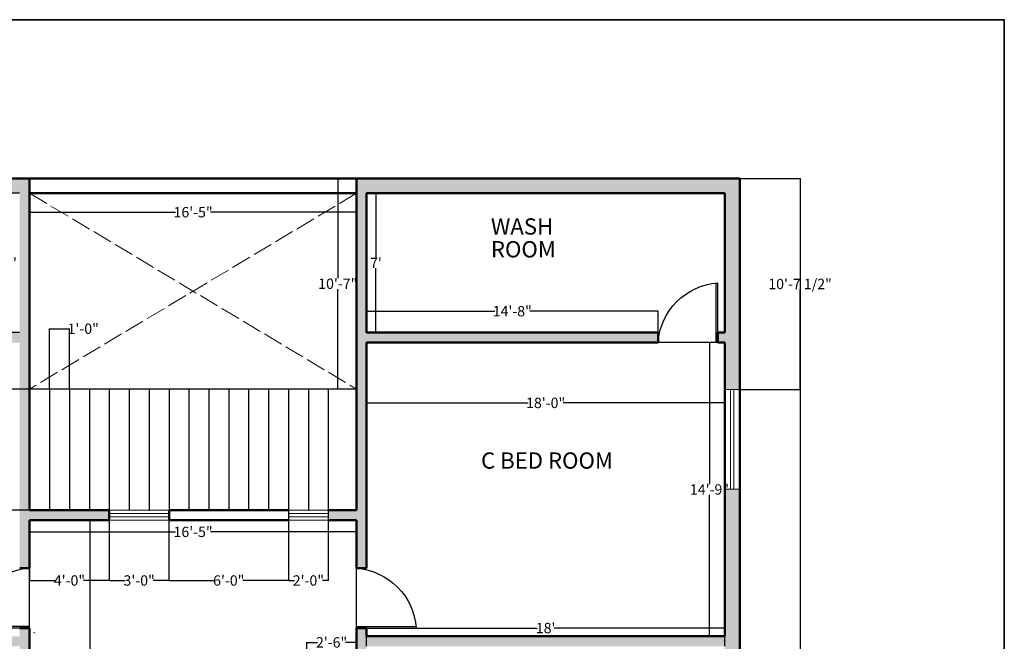
# Model space of a CAD drawing. Units: inches. Extents: x -335 to 1312, y -66 to 821.
# Tile 4 of 4: x 719 to 1312, y 446 to 821. Entities that reach past the tile are written whole.
import ezdxf

# ---------------------------------------------------------------- set-up
doc = ezdxf.new("R2010")
doc.units = ezdxf.units.IN
doc.header["$MEASUREMENT"] = 0
doc.linetypes.add('ACAD_ISO02W100', pattern=[15, 12, -3])
for name, color, linetype, lineweight in [('A-ANNO-DIMS', 2, 'Continuous', 18), ('A-ANNO-TTLB', 7, 'Continuous', 35), ('A-AREA-IDEN', 7, 'Continuous', 25), ('A-DOOR', 34, 'Continuous', 25), ('A-FLOR-OVHD', 8, 'ACAD_ISO02W100', 13), ('A-FLOR-STRS', 7, 'Continuous', 25), ('A-GLAZ', 34, 'Continuous', 18), ('A-WALL', 7, 'Continuous', 50), ('A-WALL-PATT', 252, 'Continuous', 13)]:
    doc.layers.add(name, color=color, linetype=linetype, lineweight=lineweight)
doc.styles.get("Standard").update_dxf_attribs({"font": 'arial.ttf'})
doc.dimstyles.get("Standard").update_dxf_attribs({"dimtxt": 6.25, "dimasz": 0.18, "dimexe": 0.18, "dimexo": 0.0625, "dimgap": 0.09, "dimtad": 0, "dimtih": 1, "dimtoh": 1, "dimdec": 0, "dimzin": 0, "dimdsep": 46, "dimlunit": 3, "dimtxsty": 'Standard', "dimcen": 0.09, "dimadec": 0, "dimazin": 0, "dimtfac": 1, "dimtdec": 0, "dimtofl": 0, "dimtmove": 0, "dimatfit": 3, "dimfxl": 1, "dimtolj": 1, "dimtzin": 0, "dimarcsym": 0})

# ---------------------------------------------------------------- blocks, each defined once
blk = doc.blocks.new('*D2')
at = {"layer": 'A-ANNO-DIMS', "color": 0, "lineweight": -2, "transparency": 16777216}
for p, q in [((718.49, 716.41), (713.15, 716.41)), ((713.33, 716.23), (713.33, 677.62)), ((713.33, 632.59), (713.33, 671.19)), ((718.49, 632.41), (713.15, 632.41))]:
    blk.add_line(p, q, dxfattribs=at)
at = {"layer": 'A-ANNO-DIMS', "color": 0, "transparency": 16777216}
for points in [[(713.3, 716.23), (713.36, 716.23), (713.33, 716.41)], [(713.3, 632.59), (713.36, 632.59), (713.33, 632.41)]]:
    blk.add_solid(points, dxfattribs=at)
at = {"layer": 'Defpoints', "color": 0, "transparency": 16777216}
for p in [(718.55, 716.41), (713.33, 632.41), (718.55, 632.41)]:
    blk.add_point(p, dxfattribs=at)
at = {"layer": 'A-ANNO-DIMS', "color": 0, "transparency": 16777216, "insert": (713.33, 674.41), "char_height": 6.25, "attachment_point": 5}
blk.add_mtext("\\A1;7'", dxfattribs=at)
blk = doc.blocks.new('*D18')
at = {"layer": 'A-ANNO-DIMS', "color": 0, "lineweight": -2, "transparency": 16777216}
for p, q in [((927.55, 443.47), (927.55, 454.59)), ((927.73, 454.41), (1030.45, 454.41)), ((1143.37, 454.41), (1040.65, 454.41)), ((1143.55, 443.47), (1143.55, 454.59))]:
    blk.add_line(p, q, dxfattribs=at)
at = {"layer": 'A-ANNO-DIMS', "color": 0, "transparency": 16777216}
for points in [[(927.73, 454.44), (927.73, 454.38), (927.55, 454.41)], [(1143.37, 454.44), (1143.37, 454.38), (1143.55, 454.41)]]:
    blk.add_solid(points, dxfattribs=at)
at = {"layer": 'Defpoints', "color": 0, "transparency": 16777216}
for p in [(927.55, 454.41), (927.55, 443.41), (1143.55, 443.41)]:
    blk.add_point(p, dxfattribs=at)
at = {"layer": 'A-ANNO-DIMS', "color": 0, "transparency": 16777216, "insert": (1035.55, 454.41), "char_height": 6.25, "attachment_point": 5}
blk.add_mtext("\\A1;18'", dxfattribs=at)
blk = doc.blocks.new('*D19')
at = {"layer": 'A-ANNO-DIMS', "color": 0, "lineweight": -2, "transparency": 16777216}
for p, q in [((1143.49, 626.41), (1134.12, 626.41)), ((1134.3, 626.23), (1134.3, 541.19)), ((1134.3, 449.59), (1134.3, 534.63)), ((1143.49, 449.41), (1134.12, 449.41))]:
    blk.add_line(p, q, dxfattribs=at)
at = {"layer": 'A-ANNO-DIMS', "color": 0, "transparency": 16777216}
for points in [[(1134.27, 626.23), (1134.33, 626.23), (1134.3, 626.41)], [(1134.27, 449.59), (1134.33, 449.59), (1134.3, 449.41)]]:
    blk.add_solid(points, dxfattribs=at)
at = {"layer": 'Defpoints', "color": 0, "transparency": 16777216}
for p in [(1134.3, 626.41), (1143.55, 626.41), (1143.55, 449.41)]:
    blk.add_point(p, dxfattribs=at)
at = {"layer": 'A-ANNO-DIMS', "color": 0, "transparency": 16777216, "insert": (1134.3, 537.91), "char_height": 6.25, "attachment_point": 5}
blk.add_mtext('\\A1;14\'-9"', dxfattribs=at)
blk = doc.blocks.new('*D20')
at = {"layer": 'A-ANNO-DIMS', "color": 0, "lineweight": -2, "transparency": 16777216}
for p, q in [((927.55, 632.47), (927.55, 645.55)), ((927.73, 645.37), (1004.9, 645.37)), ((1103.13, 645.37), (1025.96, 645.37)), ((1103.31, 632.47), (1103.31, 645.55))]:
    blk.add_line(p, q, dxfattribs=at)
at = {"layer": 'A-ANNO-DIMS', "color": 0, "transparency": 16777216}
for points in [[(927.73, 645.4), (927.73, 645.34), (927.55, 645.37)], [(1103.13, 645.4), (1103.13, 645.34), (1103.31, 645.37)]]:
    blk.add_solid(points, dxfattribs=at)
at = {"layer": 'Defpoints', "color": 0, "transparency": 16777216}
for p in [(927.55, 645.37), (927.55, 632.41), (1103.31, 632.41)]:
    blk.add_point(p, dxfattribs=at)
at = {"layer": 'A-ANNO-DIMS', "color": 0, "transparency": 16777216, "insert": (1015.43, 645.37), "char_height": 6.25, "attachment_point": 5}
blk.add_mtext('\\A1;14\'-8"', dxfattribs=at)
blk = doc.blocks.new('*D21')
at = {"layer": 'A-ANNO-DIMS', "color": 0, "lineweight": -2, "transparency": 16777216}
for p, q in [((927.61, 716.41), (933.44, 716.41)), ((933.26, 716.23), (933.26, 677.62)), ((933.26, 632.59), (933.26, 671.19)), ((927.61, 632.41), (933.44, 632.41))]:
    blk.add_line(p, q, dxfattribs=at)
at = {"layer": 'A-ANNO-DIMS', "color": 0, "transparency": 16777216}
for points in [[(933.23, 716.23), (933.29, 716.23), (933.26, 716.41)], [(933.23, 632.59), (933.29, 632.59), (933.26, 632.41)]]:
    blk.add_solid(points, dxfattribs=at)
at = {"layer": 'Defpoints', "color": 0, "transparency": 16777216}
for p in [(927.55, 716.41), (927.55, 632.41), (933.26, 632.41)]:
    blk.add_point(p, dxfattribs=at)
at = {"layer": 'A-ANNO-DIMS', "color": 0, "transparency": 16777216, "insert": (933.26, 674.41), "char_height": 6.25, "attachment_point": 5}
blk.add_mtext("\\A1;7'", dxfattribs=at)
blk = doc.blocks.new('*D22')
at = {"layer": 'A-ANNO-DIMS', "color": 0, "lineweight": -2, "transparency": 16777216}
for p, q in [((724.55, 519.35), (724.55, 512.18)), ((921.55, 519.35), (921.55, 512.18)), ((724.73, 512.36), (812.52, 512.36)), ((921.37, 512.36), (833.58, 512.36))]:
    blk.add_line(p, q, dxfattribs=at)
at = {"layer": 'A-ANNO-DIMS', "color": 0, "transparency": 16777216}
for points in [[(724.73, 512.39), (724.73, 512.33), (724.55, 512.36)], [(921.37, 512.39), (921.37, 512.33), (921.55, 512.36)]]:
    blk.add_solid(points, dxfattribs=at)
at = {"layer": 'Defpoints', "color": 0, "transparency": 16777216}
for p in [(724.55, 519.41), (921.55, 519.41), (921.55, 512.36)]:
    blk.add_point(p, dxfattribs=at)
at = {"layer": 'A-ANNO-DIMS', "color": 0, "transparency": 16777216, "insert": (823.05, 512.36), "char_height": 6.25, "attachment_point": 5}
blk.add_mtext('\\A1;16\'-5"', dxfattribs=at)
blk = doc.blocks.new('*D23')
at = {"layer": 'A-ANNO-DIMS', "color": 0, "lineweight": -2, "transparency": 16777216}
for p, q in [((724.55, 716.35), (724.55, 704.82)), ((921.55, 716.35), (921.55, 704.82)), ((724.73, 705), (812.52, 705)), ((921.37, 705), (833.58, 705))]:
    blk.add_line(p, q, dxfattribs=at)
at = {"layer": 'A-ANNO-DIMS', "color": 0, "transparency": 16777216}
for points in [[(724.73, 705.03), (724.73, 704.97), (724.55, 705)], [(921.37, 705.03), (921.37, 704.97), (921.55, 705)]]:
    blk.add_solid(points, dxfattribs=at)
at = {"layer": 'Defpoints', "color": 0, "transparency": 16777216}
for p in [(724.55, 716.41), (921.55, 716.41), (724.55, 705)]:
    blk.add_point(p, dxfattribs=at)
at = {"layer": 'A-ANNO-DIMS', "color": 0, "transparency": 16777216, "insert": (823.05, 705), "char_height": 6.25, "attachment_point": 5}
blk.add_mtext('\\A1;16\'-5"', dxfattribs=at)
blk = doc.blocks.new('*D24')
at = {"layer": 'A-ANNO-DIMS', "color": 0, "lineweight": -2, "transparency": 16777216}
for p, q in [((921.49, 725.41), (910.09, 725.41)), ((910.27, 725.23), (910.27, 665.19)), ((910.27, 598.59), (910.27, 658.63)), ((921.49, 598.41), (910.09, 598.41))]:
    blk.add_line(p, q, dxfattribs=at)
at = {"layer": 'A-ANNO-DIMS', "color": 0, "transparency": 16777216}
for points in [[(910.24, 725.23), (910.3, 725.23), (910.27, 725.41)], [(910.24, 598.59), (910.3, 598.59), (910.27, 598.41)]]:
    blk.add_solid(points, dxfattribs=at)
at = {"layer": 'Defpoints', "color": 0, "transparency": 16777216}
for p in [(921.55, 725.41), (910.27, 598.41), (921.55, 598.41)]:
    blk.add_point(p, dxfattribs=at)
at = {"layer": 'A-ANNO-DIMS', "color": 0, "transparency": 16777216, "insert": (910.27, 661.91), "char_height": 6.25, "attachment_point": 5}
blk.add_mtext('\\A1;10\'-7"', dxfattribs=at)
blk = doc.blocks.new('WIN-60IN')
for p, q in [((9, 60), (0, 60)), ((0, 60), (0, 0)), ((3.5, 60), (3.5, 0)), ((5.5, 60), (5.5, 0)), ((9, 0), (9, 60)), ((0, 0), (9, 0))]:
    blk.add_line(p, q)
blk = doc.blocks.new('DOOR-SWING-36IN')
for p, q in [((0, 0), (0, 35.94)), ((1, 0), (1, 35.86)), ((0, 0), (36, 0))]:
    blk.add_line(p, q)
blk.add_arc((-2.68, -2.74), 38.78, 4.05456, 86.03519)
blk = doc.blocks.new('*D32')
at = {"layer": 'A-ANNO-DIMS', "color": 0, "lineweight": -2, "transparency": 16777216}
for p, q in [((927.55, 626.35), (927.55, 589.88)), ((1143.55, 626.35), (1143.55, 589.88)), ((927.73, 590.06), (1025.02, 590.06)), ((1143.37, 590.06), (1046.08, 590.06))]:
    blk.add_line(p, q, dxfattribs=at)
at = {"layer": 'A-ANNO-DIMS', "color": 0, "transparency": 16777216}
for points in [[(927.73, 590.09), (927.73, 590.03), (927.55, 590.06)], [(1143.37, 590.09), (1143.37, 590.03), (1143.55, 590.06)]]:
    blk.add_solid(points, dxfattribs=at)
at = {"layer": 'Defpoints', "color": 0, "transparency": 16777216}
for p in [(927.55, 626.41), (1143.55, 626.41), (927.55, 590.06)]:
    blk.add_point(p, dxfattribs=at)
at = {"layer": 'A-ANNO-DIMS', "color": 0, "transparency": 16777216, "insert": (1035.55, 590.06), "char_height": 6.25, "attachment_point": 5}
blk.add_mtext('\\A1;18\'-0"', dxfattribs=at)
blk = doc.blocks.new('*D34')
at = {"layer": 'A-ANNO-DIMS', "color": 0, "lineweight": -2, "transparency": 16777216}
for p, q in [((736.49, 598.41), (700.02, 598.41)), ((700.2, 598.23), (700.2, 565.19)), ((700.2, 525.59), (700.2, 558.63)), ((736.49, 525.41), (700.02, 525.41))]:
    blk.add_line(p, q, dxfattribs=at)
at = {"layer": 'A-ANNO-DIMS', "color": 0, "transparency": 16777216}
for points in [[(700.17, 598.23), (700.23, 598.23), (700.2, 598.41)], [(700.17, 525.59), (700.23, 525.59), (700.2, 525.41)]]:
    blk.add_solid(points, dxfattribs=at)
at = {"layer": 'Defpoints', "color": 0, "transparency": 16777216}
for p in [(700.2, 598.41), (736.55, 598.41), (736.55, 525.41)]:
    blk.add_point(p, dxfattribs=at)
at = {"layer": 'A-ANNO-DIMS', "color": 0, "transparency": 16777216, "insert": (700.2, 561.91), "char_height": 6.25, "attachment_point": 5}
blk.add_mtext('\\A1;6\'-1"', dxfattribs=at)
blk = doc.blocks.new('*D40')
at = {"layer": 'A-ANNO-DIMS', "color": 0, "lineweight": -2, "transparency": 16777216}
for p, q in [((1152.61, 725.41), (1189.08, 725.41)), ((1188.9, 725.23), (1188.9, 665.06)), ((1188.9, 598.25), (1188.9, 658.42)), ((1152.61, 598.07), (1189.08, 598.07))]:
    blk.add_line(p, q, dxfattribs=at)
at = {"layer": 'A-ANNO-DIMS', "color": 0, "transparency": 16777216}
for points in [[(1188.87, 725.23), (1188.93, 725.23), (1188.9, 725.41)], [(1188.87, 598.25), (1188.93, 598.25), (1188.9, 598.07)]]:
    blk.add_solid(points, dxfattribs=at)
at = {"layer": 'Defpoints', "color": 0, "transparency": 16777216}
for p in [(1152.55, 725.41), (1152.55, 598.07), (1188.9, 598.07)]:
    blk.add_point(p, dxfattribs=at)
at = {"layer": 'A-ANNO-DIMS', "color": 0, "transparency": 16777216, "insert": (1188.9, 661.74), "char_height": 6.25, "attachment_point": 5}
blk.add_mtext('\\A1;10\'-7 1/2"', dxfattribs=at)
blk = doc.blocks.new('*D42')
at = {"layer": 'A-ANNO-DIMS', "color": 0, "lineweight": -2, "transparency": 16777216}
for p, q in [((1152.61, 725.41), (1189.08, 725.41)), ((1188.9, 725.23), (1188.9, 368.69)), ((1188.9, 5.59), (1188.9, 362.13)), ((1152.61, 5.41), (1189.08, 5.41))]:
    blk.add_line(p, q, dxfattribs=at)
at = {"layer": 'A-ANNO-DIMS', "color": 0, "transparency": 16777216}
for points in [[(1188.87, 725.23), (1188.93, 725.23), (1188.9, 725.41)], [(1188.87, 5.59), (1188.93, 5.59), (1188.9, 5.41)]]:
    blk.add_solid(points, dxfattribs=at)
at = {"layer": 'Defpoints', "color": 0, "transparency": 16777216}
for p in [(1152.55, 725.41), (1188.9, 725.41), (1152.55, 5.41)]:
    blk.add_point(p, dxfattribs=at)
at = {"layer": 'A-ANNO-DIMS', "color": 0, "transparency": 16777216, "insert": (1188.9, 365.41), "char_height": 6.25, "attachment_point": 5}
blk.add_mtext('\\A1;60\'-0"', dxfattribs=at)
blk = doc.blocks.new('*D45')
at = {"layer": 'A-ANNO-DIMS', "color": 0, "lineweight": -2, "transparency": 16777216}
for p, q in [((891.55, 409.47), (891.55, 445.94)), ((891.73, 445.76), (898.1, 445.76)), ((921.37, 445.76), (915, 445.76)), ((921.55, 409.47), (921.55, 445.94))]:
    blk.add_line(p, q, dxfattribs=at)
at = {"layer": 'A-ANNO-DIMS', "color": 0, "transparency": 16777216}
for points in [[(891.73, 445.79), (891.73, 445.73), (891.55, 445.76)], [(921.37, 445.79), (921.37, 445.73), (921.55, 445.76)]]:
    blk.add_solid(points, dxfattribs=at)
at = {"layer": 'Defpoints', "color": 0, "transparency": 16777216}
for p in [(921.55, 445.76), (891.55, 409.41), (921.55, 409.41)]:
    blk.add_point(p, dxfattribs=at)
at = {"layer": 'A-ANNO-DIMS', "color": 0, "transparency": 16777216, "insert": (906.55, 445.76), "char_height": 6.25, "attachment_point": 5}
blk.add_mtext('\\A1;2\'-6"', dxfattribs=at)
blk = doc.blocks.new('*D47')
at = {"layer": 'A-ANNO-DIMS', "color": 0, "lineweight": -2, "transparency": 16777216}
for p, q in [((724.61, 519.41), (761.08, 519.41)), ((760.9, 519.23), (760.9, 404.69)), ((760.9, 283.59), (760.9, 398.13)), ((724.61, 283.41), (761.08, 283.41))]:
    blk.add_line(p, q, dxfattribs=at)
at = {"layer": 'A-ANNO-DIMS', "color": 0, "transparency": 16777216}
for points in [[(760.87, 519.23), (760.93, 519.23), (760.9, 519.41)], [(760.87, 283.59), (760.93, 283.59), (760.9, 283.41)]]:
    blk.add_solid(points, dxfattribs=at)
at = {"layer": 'Defpoints', "color": 0, "transparency": 16777216}
for p in [(724.55, 519.41), (724.55, 283.41), (760.9, 283.41)]:
    blk.add_point(p, dxfattribs=at)
at = {"layer": 'A-ANNO-DIMS', "color": 0, "transparency": 16777216, "insert": (760.9, 401.41), "char_height": 6.25, "attachment_point": 5}
blk.add_mtext('\\A1;19\'-8"', dxfattribs=at)
blk = doc.blocks.new('*D48')
at = {"layer": 'A-ANNO-DIMS', "color": 0, "lineweight": -2, "transparency": 16777216}
for p, q in [((772.54, 519.35), (772.54, 482.88)), ((808.54, 519.35), (808.54, 482.88)), ((772.72, 483.06), (782.14, 483.06)), ((808.36, 483.06), (798.93, 483.06))]:
    blk.add_line(p, q, dxfattribs=at)
at = {"layer": 'A-ANNO-DIMS', "color": 0, "transparency": 16777216}
for points in [[(772.72, 483.09), (772.72, 483.03), (772.54, 483.06)], [(808.36, 483.09), (808.36, 483.03), (808.54, 483.06)]]:
    blk.add_solid(points, dxfattribs=at)
at = {"layer": 'Defpoints', "color": 0, "transparency": 16777216}
for p in [(772.54, 519.41), (808.54, 519.41), (772.54, 483.06)]:
    blk.add_point(p, dxfattribs=at)
at = {"layer": 'A-ANNO-DIMS', "color": 0, "transparency": 16777216, "insert": (790.54, 483.06), "char_height": 6.25, "attachment_point": 5}
blk.add_mtext('\\A1;3\'-0"', dxfattribs=at)
blk = doc.blocks.new('*D49')
at = {"layer": 'A-ANNO-DIMS', "color": 0, "lineweight": -2, "transparency": 16777216}
for p, q in [((880.55, 519.35), (880.55, 482.88)), ((904.55, 519.35), (904.55, 482.88)), ((880.73, 483.06), (884.1, 483.06)), ((904.37, 483.06), (901, 483.06))]:
    blk.add_line(p, q, dxfattribs=at)
at = {"layer": 'A-ANNO-DIMS', "color": 0, "transparency": 16777216}
for points in [[(880.73, 483.09), (880.73, 483.03), (880.55, 483.06)], [(904.37, 483.09), (904.37, 483.03), (904.55, 483.06)]]:
    blk.add_solid(points, dxfattribs=at)
at = {"layer": 'Defpoints', "color": 0, "transparency": 16777216}
for p in [(880.55, 519.41), (904.55, 519.41), (880.55, 483.06)]:
    blk.add_point(p, dxfattribs=at)
at = {"layer": 'A-ANNO-DIMS', "color": 0, "transparency": 16777216, "insert": (892.55, 483.06), "char_height": 6.25, "attachment_point": 5}
blk.add_mtext('\\A1;2\'-0"', dxfattribs=at)
blk = doc.blocks.new('*D50')
at = {"layer": 'A-ANNO-DIMS', "color": 0, "lineweight": -2, "transparency": 16777216}
for p, q in [((724.55, 519.35), (724.55, 482.88)), ((772.54, 519.35), (772.54, 482.88)), ((724.73, 483.06), (740.02, 483.06)), ((772.36, 483.06), (757.07, 483.06))]:
    blk.add_line(p, q, dxfattribs=at)
at = {"layer": 'A-ANNO-DIMS', "color": 0, "transparency": 16777216}
for points in [[(724.73, 483.09), (724.73, 483.03), (724.55, 483.06)], [(772.36, 483.09), (772.36, 483.03), (772.54, 483.06)]]:
    blk.add_solid(points, dxfattribs=at)
at = {"layer": 'Defpoints', "color": 0, "transparency": 16777216}
for p in [(724.55, 519.41), (772.54, 519.41), (724.55, 483.06)]:
    blk.add_point(p, dxfattribs=at)
at = {"layer": 'A-ANNO-DIMS', "color": 0, "transparency": 16777216, "insert": (748.54, 483.06), "char_height": 6.25, "attachment_point": 5}
blk.add_mtext('\\A1;4\'-0"', dxfattribs=at)
blk = doc.blocks.new('*D51')
at = {"layer": 'A-ANNO-DIMS', "color": 0, "lineweight": -2, "transparency": 16777216}
for p, q in [((808.54, 519.35), (808.54, 482.88)), ((880.55, 519.35), (880.55, 482.88)), ((808.72, 483.06), (836.13, 483.06)), ((880.37, 483.06), (852.96, 483.06))]:
    blk.add_line(p, q, dxfattribs=at)
at = {"layer": 'A-ANNO-DIMS', "color": 0, "transparency": 16777216}
for points in [[(808.72, 483.09), (808.72, 483.03), (808.54, 483.06)], [(880.37, 483.09), (880.37, 483.03), (880.55, 483.06)]]:
    blk.add_solid(points, dxfattribs=at)
at = {"layer": 'Defpoints', "color": 0, "transparency": 16777216}
for p in [(808.54, 519.41), (880.55, 519.41), (808.54, 483.06)]:
    blk.add_point(p, dxfattribs=at)
at = {"layer": 'A-ANNO-DIMS', "color": 0, "transparency": 16777216, "insert": (844.55, 483.06), "char_height": 6.25, "attachment_point": 5}
blk.add_mtext('\\A1;6\'-0"', dxfattribs=at)
blk = doc.blocks.new('*D52')
at = {"layer": 'A-ANNO-DIMS', "color": 0, "lineweight": -2, "transparency": 16777216}
for p, q in [((736.55, 598.47), (736.55, 634.94)), ((736.73, 634.76), (748.37, 634.76)), ((748.55, 598.47), (748.55, 634.94)), ((748.55, 634.76), (748.73, 634.76))]:
    blk.add_line(p, q, dxfattribs=at)
at = {"layer": 'A-ANNO-DIMS', "color": 0, "transparency": 16777216}
for points in [[(736.73, 634.79), (736.73, 634.73), (736.55, 634.76)], [(748.37, 634.79), (748.37, 634.73), (748.55, 634.76)]]:
    blk.add_solid(points, dxfattribs=at)
at = {"layer": 'Defpoints', "color": 0, "transparency": 16777216}
for p in [(748.55, 634.76), (736.55, 598.41), (748.55, 598.41)]:
    blk.add_point(p, dxfattribs=at)
at = {"layer": 'A-ANNO-DIMS', "color": 0, "transparency": 16777216, "insert": (756.83, 634.76), "char_height": 6.25, "attachment_point": 5}
blk.add_mtext('\\A1;1\'-0"', dxfattribs=at)
blk = doc.blocks.new('*D62')
at = {"layer": 'A-ANNO-DIMS', "color": 0, "lineweight": -2, "transparency": 16777216}
for p, q in [((683.21, 495.57), (683.39, 495.57)), ((683.39, 495.57), (699.72, 479.25)), ((727.2, 451.73), (727.38, 451.73)), ((727.29, 451.64), (727.29, 451.82))]:
    blk.add_line(p, q, dxfattribs=at)
at = {"layer": 'A-ANNO-DIMS', "color": 0, "transparency": 16777216}
blk.add_solid([(699.74, 479.27), (699.7, 479.23), (699.85, 479.13)], dxfattribs=at)
at = {"layer": 'Defpoints', "color": 0, "transparency": 16777216}
for p in [(699.85, 479.13), (727.29, 451.73)]:
    blk.add_point(p, dxfattribs=at)
at = {"layer": 'A-ANNO-DIMS', "color": 0, "transparency": 16777216, "insert": (665.11, 495.57), "char_height": 6.25, "attachment_point": 5}
blk.add_mtext('\\A1;3X R3\'-3"', dxfattribs=at)

msp = doc.modelspace()

# ---------------------------------------------------------------- hatches: boundary and pattern name
at = {"layer": 'A-WALL-PATT'}
h = msp.add_hatch(color=256, dxfattribs=at)
h.dxf.hatch_style = 1
h.paths.add_polyline_path([(561.55, 92.41), (552.55, 92.41), (552.55, 5.41), (724.55, 5.41), (724.55, 84.41), (727.55, 84.41), (727.55, 93.41), (724.55, 93.41), (724.55, 158.41), (712.55, 158.41), (712.55, 152.41), (718.55, 152.41), (718.55, 14.41), (561.55, 14.41)])
h.paths.add_polyline_path([(561.55, 254.41), (657.55, 254.41), (657.55, 200.41), (663.55, 200.41), (663.55, 254.41), (724.55, 254.41), (724.55, 278.41), (728.55, 278.41), (728.55, 283.41), (724.55, 283.41), (724.55, 295.41), (718.55, 295.41), (718.55, 260.41), (561.55, 260.41), (561.55, 318.41), (552.55, 318.41), (552.55, 152.41), (561.55, 152.41), (676.55, 152.41), (676.55, 158.41), (663.55, 158.41), (663.55, 164.41), (657.55, 164.41), (657.55, 158.41), (561.55, 158.41)])
h.paths.add_polyline_path([(561.55, 443.41), (634.55, 443.41), (634.55, 384.41), (634.55, 378.41), (676.55, 378.41), (676.55, 384.41), (640.55, 384.41), (640.55, 443.41), (718.55, 443.41), (718.55, 384.41), (712.55, 384.41), (712.55, 378.41), (718.55, 378.41), (718.55, 331.41), (724.55, 331.41), (724.55, 454.41), (718.55, 454.41), (718.55, 449.41), (561.55, 449.41), (561.55, 535.84), (552.55, 535.84), (552.55, 378.41), (561.55, 378.41), (598.55, 378.41), (598.55, 384.41), (561.55, 384.41)])
h.paths.add_polyline_path([(724.55, 725.41), (552.55, 725.41), (552.55, 595.84), (561.55, 595.84), (561.55, 626.41), (566.55, 626.41), (566.55, 632.41), (561.55, 632.41), (561.55, 716.41), (718.55, 716.41), (718.55, 632.41), (602.55, 632.41), (602.55, 626.41), (718.55, 626.41), (718.55, 490.41), (724.55, 490.41), (724.55, 519.41), (772.54, 519.41), (772.56, 525.41), (724.55, 525.41)])
h.paths.add_polyline_path([(927.55, 716.41), (1143.55, 716.41), (1143.55, 632.41), (1139.31, 632.41), (1139.31, 626.41), (1143.55, 626.41), (1143.55, 598.07), (1152.55, 598.07), (1152.55, 725.41), (921.55, 725.41), (921.55, 598.41), (921.55, 525.41), (904.55, 525.41), (904.55, 519.41), (921.55, 519.41), (921.55, 490.41), (927.55, 490.41), (927.55, 626.41), (1103.31, 626.41), (1103.31, 632.41), (927.55, 632.41)])
h.paths.add_polyline_path([(1152.55, 538.07), (1143.55, 538.07), (1143.55, 449.41), (927.55, 449.41), (927.55, 454.41), (921.55, 454.41), (921.55, 283.41), (764.57, 283.41), (764.55, 278.41), (921.55, 278.41), (921.55, 261.75), (927.55, 261.75), (927.55, 443.41), (1143.55, 443.41), (1143.55, 284.87), (1152.55, 284.87)])
h.paths.add_polyline_path([(930.55, 206.41), (1143.55, 206.41), (1143.55, 215.41), (927.55, 215.41), (927.55, 225.75), (921.55, 225.75), (921.55, 93.41), (857.84, 93.41), (857.84, 84.41), (930.55, 84.41)])
h.paths.add_polyline_path([(1152.55, 206.41), (1143.55, 206.41), (1143.55, 5.41), (1152.55, 5.41)])
h.paths.add_polyline_path([(797.84, 93.41), (763.55, 93.41), (763.55, 84.41), (797.84, 84.41)])

# ---------------------------------------------------------------- linework, layer by layer
at = {"layer": 'A-ANNO-TTLB'}
msp.add_lwpolyline([(405.31, 821.01), (1312, 821.01), (1312, -66.33), (405.31, -66.33)], close=True, dxfattribs=at)
at = {"layer": 'A-FLOR-OVHD'}
for p, q in [((724.55, 716.41), (921.55, 598.41)), ((921.55, 716.41), (724.55, 598.41))]:
    msp.add_line(p, q, dxfattribs=at)
at = {"layer": 'A-FLOR-STRS'}
for p, q in [((921.55, 598.41), (724.55, 598.41)), ((736.55, 598.41), (736.55, 525.41)), ((748.55, 598.41), (748.55, 525.41)), ((760.55, 598.41), (760.55, 525.41)), ((772.55, 598.41), (772.55, 525.41)), ((784.55, 598.41), (784.55, 525.41)), ((796.55, 598.41), (796.55, 525.41)), ((808.55, 598.41), (808.55, 525.41)), ((820.55, 598.41), (820.55, 525.41)), ((832.55, 598.41), (832.55, 525.41)), ((844.55, 598.41), (844.55, 525.41)), ((856.55, 598.41), (856.55, 525.41)), ((868.55, 598.41), (868.55, 525.41)), ((880.55, 598.41), (880.55, 519.41)), ((892.55, 598.41), (892.55, 525.41)), ((904.55, 598.41), (904.55, 519.41))]:
    msp.add_line(p, q, dxfattribs=at)
at = {"layer": 'A-GLAZ'}
for p, q in [((772.55, 523.38), (808.57, 523.38)), ((772.56, 525.38), (808.57, 525.41)), ((880.55, 525.41), (904.55, 525.41)), ((880.55, 523.38), (904.55, 523.38)), ((808.57, 519.41), (772.54, 519.38)), ((772.55, 521.38), (808.57, 521.38)), ((880.55, 521.38), (904.55, 521.38)), ((904.55, 519.41), (880.55, 519.41))]:
    msp.add_line(p, q, dxfattribs=at)
at = {"layer": 'A-WALL'}
for p, q in [((1152.55, 725.41), (552.55, 725.41)), ((724.55, 725.41), (724.55, 525.41)), ((921.55, 725.41), (921.55, 598.41)), ((1152.55, 245.41), (1152.55, 725.41)), ((921.55, 716.41), (724.55, 716.41)), ((1143.55, 716.41), (927.55, 716.41)), ((927.55, 716.41), (927.55, 632.41)), ((1143.55, 632.41), (1143.55, 716.41)), ((1103.31, 632.41), (927.55, 632.41)), ((1103.31, 632.41), (1103.31, 626.41)), ((1143.55, 632.41), (1139.31, 632.41)), ((1139.31, 632.41), (1139.31, 626.41)), ((927.55, 626.41), (927.55, 490.41)), ((1103.31, 626.41), (927.55, 626.41)), ((1143.55, 626.41), (1139.31, 626.41)), ((1143.55, 449.41), (1143.55, 626.41)), ((921.55, 598.41), (921.55, 525.41)), ((724.55, 525.41), (772.55, 525.41)), ((772.56, 525.38), (772.54, 519.38)), ((808.55, 525.41), (880.55, 525.41)), ((808.57, 525.41), (808.57, 519.41)), ((904.55, 525.41), (921.55, 525.41)), ((724.55, 519.41), (772.54, 519.41)), ((724.55, 519.41), (724.55, 490.41)), ((808.54, 519.41), (880.55, 519.41)), ((904.55, 519.41), (921.55, 519.41)), ((921.55, 519.41), (921.55, 490.41)), ((718.55, 490.41), (724.55, 490.41)), ((921.55, 490.41), (927.55, 490.41)), ((718.55, 454.41), (724.55, 454.41)), ((724.55, 454.41), (724.55, 331.41)), ((921.55, 454.41), (927.55, 454.41)), ((921.55, 454.41), (921.55, 283.41)), ((927.55, 454.41), (927.55, 449.41)), ((1143.55, 449.41), (927.55, 449.41))]:
    msp.add_line(p, q, dxfattribs=at)

# ---------------------------------------------------------------- block references
at = {"layer": 'A-DOOR', "extrusion": (0, 0, -1), "zscale": -1}
msp.add_blockref('DOOR-SWING-36IN', (-1139.31, 626.41), dxfattribs=at)
at = {"layer": 'A-DOOR', "rotation": 89.99999999999935}
msp.add_blockref('DOOR-SWING-36IN', (724.55, 454.41), dxfattribs=at)
at = {"layer": 'A-DOOR', "extrusion": (0, 0, -1), "zscale": -1, "rotation": 90.00000000000047}
msp.add_blockref('DOOR-SWING-36IN', (-921.55, 454.41), dxfattribs=at)
at = {"layer": 'A-GLAZ'}
msp.add_blockref('WIN-60IN', (1143.55, 538.07), dxfattribs=at)

# ---------------------------------------------------------------- texts
at = {"layer": 'A-AREA-IDEN'}
for s, p in [('WASH ', (1002.56, 691.52)), ('ROOM', (1002.56, 677.76)), ('C BED ROOM', (996.64, 550.44))]:
    msp.add_text(s, height=9.789, dxfattribs=at).set_placement(p)

# ---------------------------------------------------------------- dimensions: what is measured, and where the dimension line sits
at = {"layer": 'A-ANNO-DIMS'}
for base, p1, p2, angle, override, picture, middle in [((910.27, 598.41), (921.55, 725.41), (921.55, 598.41), 90, {"dimclrd": 0, "dimclre": 0, "dimclrt": 0}, '*D24', (910.27, 661.91)), ((1188.9, 598.07), (1152.55, 725.41), (1152.55, 598.07), 270, {"dimdec": 1, "dimlfac": 1, "dimrnd": 0, "dimzin": 1, "dimdsep": 46, "dimlunit": 4, "dimfrac": 2}, '*D40', (1188.9, 661.74)), ((1188.9, 725.41), (1152.55, 5.41), (1152.55, 725.41), 90, {"dimdec": 1, "dimlfac": 1, "dimrnd": 0, "dimzin": 1, "dimdsep": 46, "dimlunit": 4, "dimfrac": 2}, '*D42', (1188.9, 365.41)), ((713.33, 632.41), (718.55, 716.41), (718.55, 632.41), 90, {"dimclrd": 0, "dimclre": 0, "dimclrt": 0}, '*D2', (713.33, 674.41)), ((933.26, 632.41), (927.55, 716.41), (927.55, 632.41), 90, {"dimclrd": 0, "dimclre": 0, "dimclrt": 0}, '*D21', (933.26, 674.41)), ((927.55, 590.06), (1143.55, 626.41), (927.55, 626.41), 180, {"dimdec": 1, "dimlfac": 1, "dimrnd": 0, "dimzin": 1, "dimdsep": 46, "dimlunit": 4, "dimfrac": 2}, '*D32', (1035.55, 590.06)), ((1134.3, 626.41), (1143.55, 449.41), (1143.55, 626.41), 90, {"dimclrd": 0, "dimclre": 0, "dimclrt": 0}, '*D19', (1134.3, 537.91)), ((700.2, 598.41), (736.55, 525.41), (736.55, 598.41), 90, {"dimdec": 1, "dimlfac": 1, "dimrnd": 0, "dimzin": 1, "dimdsep": 46, "dimlunit": 4, "dimfrac": 2}, '*D34', (700.2, 561.91)), ((760.9, 283.41), (724.55, 519.41), (724.55, 283.41), 270, {"dimdec": 1, "dimlfac": 1, "dimrnd": 0, "dimzin": 1, "dimdsep": 46, "dimlunit": 4, "dimfrac": 2}, '*D47', (760.9, 401.41)), ((724.55, 483.06), (772.54, 519.41), (724.55, 519.41), 180, {"dimdec": 1, "dimlfac": 1, "dimrnd": 0, "dimzin": 1, "dimdsep": 46, "dimlunit": 4, "dimfrac": 2}, '*D50', (748.54, 483.06)), ((772.54, 483.06), (808.54, 519.41), (772.54, 519.41), 180, {"dimdec": 1, "dimlfac": 1, "dimrnd": 0, "dimzin": 1, "dimdsep": 46, "dimlunit": 4, "dimfrac": 2}, '*D48', (790.54, 483.06)), ((808.54, 483.06), (880.55, 519.41), (808.54, 519.41), 180, {"dimdec": 1, "dimlfac": 1, "dimrnd": 0, "dimzin": 1, "dimdsep": 46, "dimlunit": 4, "dimfrac": 2}, '*D51', (844.55, 483.06)), ((880.55, 483.06), (904.55, 519.41), (880.55, 519.41), 180, {"dimdec": 1, "dimlfac": 1, "dimrnd": 0, "dimzin": 1, "dimdsep": 46, "dimlunit": 4, "dimfrac": 2}, '*D49', (892.55, 483.06))]:
    dim = msp.add_linear_dim(base=base, p1=p1, p2=p2, angle=angle, dimstyle='Standard', override=override, dxfattribs=at)
    dim.commit()
    dim.dimension.update_dxf_attribs({"geometry": picture, "text_midpoint": middle})
for base, p1, p2, override, picture, middle in [((724.55, 705), (921.55, 716.41), (724.55, 716.41), {"dimclrd": 0, "dimclre": 0, "dimclrt": 0}, '*D23', (823.05, 705)), ((927.55, 645.37), (1103.31, 632.41), (927.55, 632.41), {"dimclrd": 0, "dimclre": 0, "dimclrt": 0}, '*D20', (1015.43, 645.37)), ((748.55, 634.76), (736.55, 598.41), (748.55, 598.41), {"dimdec": 1, "dimlfac": 1, "dimrnd": 0, "dimzin": 1, "dimdsep": 46, "dimlunit": 4, "dimfrac": 2}, '*D52', (756.83, 634.76)), ((921.55, 512.36), (724.55, 519.41), (921.55, 519.41), {"dimclrd": 0, "dimclre": 0, "dimclrt": 0}, '*D22', (823.05, 512.36)), ((927.55, 454.41), (1143.55, 443.41), (927.55, 443.41), {"dimclrd": 0, "dimclre": 0, "dimclrt": 0}, '*D18', (1035.55, 454.41)), ((921.55, 445.76), (891.55, 409.41), (921.55, 409.41), {"dimdec": 1, "dimlfac": 1, "dimrnd": 0, "dimzin": 1, "dimdsep": 46, "dimlunit": 4, "dimfrac": 2}, '*D45', (906.55, 445.76))]:
    dim = msp.add_linear_dim(base=base, p1=p1, p2=p2, dimstyle='Standard', override=override, dxfattribs=at)
    dim.commit()
    dim.dimension.update_dxf_attribs({"geometry": picture, "text_midpoint": middle})
dim = msp.add_radius_dim(center=(727.29, 451.73), mpoint=(699.85, 479.13), text='3X <>', dimstyle='Standard', override={"dimdec": 1, "dimlfac": 1, "dimrnd": 0, "dimzin": 1, "dimdsep": 46, "dimlunit": 4, "dimfrac": 2}, dxfattribs=at)
dim.commit()
dim.dimension.update_dxf_attribs({"geometry": '*D62', "text_midpoint": (665.11, 495.57), "dimtype": 164})

doc.saveas('drawing.dxf')
